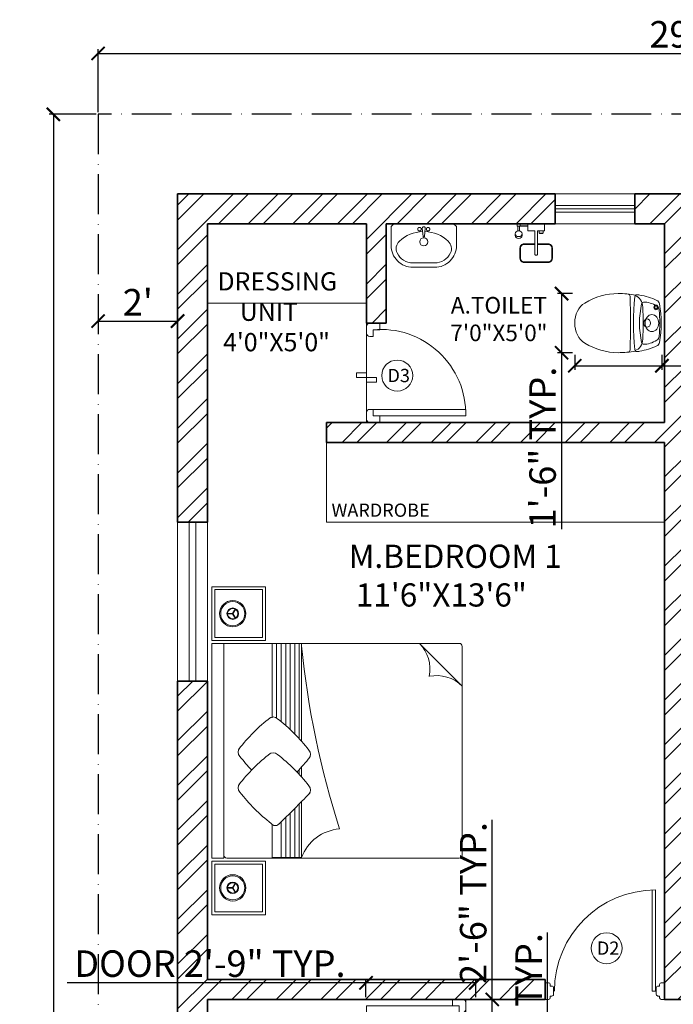
# Model space of a CAD drawing. Units: inches. Extents: x -15 to 1053, y -1 to 793.
# Tile 7 of 8: x 595 to 793, y 496 to 793. Entities that reach past the tile are written whole.
import ezdxf

# ---------------------------------------------------------------- set-up
doc = ezdxf.new("R2010")
doc.units = ezdxf.units.IN
doc.linetypes.add('ACAD_ISO10W100', pattern=[18, 12, -3, 0, -3])
for name, color, linetype, lineweight in [('00 FURNITURE', 15, 'Continuous', 15), ('A-ANNO-DIMS', 2, 'Continuous', 18), ('A-ANNO-TEXT', 7, 'Continuous', 18), ('A-AREA-IDEN', 7, 'Continuous', 18), ('A-DOOR', 4, 'Continuous', 18), ('A-FLOR-CASE', 5, 'Continuous', 18), ('A-FLOR-FIXT', 8, 'Continuous', 13), ('A-FURN', 8, 'Continuous', 13), ('A-GLAZ', 4, 'Continuous', 18), ('A-WALL', 7, 'Continuous', 35), ('A-WALL-PATT', 8, 'Continuous', 13), ('A_FUR 1', 5, 'Continuous', 5), ('C-PROP', 1, 'ACAD_ISO10W100', 25)]:
    doc.layers.add(name, color=color, linetype=linetype, lineweight=lineweight)
doc.styles.add('1-100DIM', font='txt', dxfattribs={"height": 0.3})
doc.styles.get("Standard").update_dxf_attribs({"font": 'arial.ttf'})
doc.dimstyles.new('ISO-25', dxfattribs={"dimtxt": 8, "dimasz": 4, "dimexe": 1.25, "dimexo": 0.625, "dimtad": 1, "dimdec": 0, "dimlunit": 4, "dimtxsty": 'Standard', "dimblk": 'ARCHTICK', "dimcen": 3, "dimadec": 0, "dimazin": 0, "dimtfac": 1, "dimtdec": 0, "dimtmove": 0, "dimatfit": 3, "dimldrblk": 'ARCHTICK', "dimfxl": 1, "dimarcsym": 0})

# ---------------------------------------------------------------- blocks, each defined once
blk = doc.blocks.new('_ArchTick')
at = {"color": 0, "linetype": 'ByBlock', "const_width": 0.15}
blk.add_lwpolyline([(-0.5, -0.5), (0.5, 0.5)], dxfattribs=at)
blk = doc.blocks.new('*D18')
at = {"layer": 'A-ANNO-DIMS', "color": 0, "lineweight": -2, "transparency": 16777216}
for p, q in [((619.07, 765.39), (619.07, 784.39)), ((967.07, 765.39), (967.07, 784.39)), ((619.07, 783.14), (967.07, 783.14))]:
    blk.add_line(p, q, dxfattribs=at)
at = {"layer": 'Defpoints', "color": 0, "transparency": 16777216}
for p in [(967.07, 783.14), (619.07, 764.76), (967.07, 764.76)]:
    blk.add_point(p, dxfattribs=at)
at = {"layer": 'A-ANNO-DIMS', "color": 0, "lineweight": -2, "transparency": 16777216, "xscale": 4, "yscale": 4, "zscale": 4, "rotation": 180}
blk.add_blockref('_ArchTick', (619.07, 783.14), dxfattribs=at)
at = {"layer": 'A-ANNO-DIMS', "color": 0, "lineweight": -2, "transparency": 16777216, "xscale": 4, "yscale": 4, "zscale": 4}
blk.add_blockref('_ArchTick', (967.07, 783.14), dxfattribs=at)
at = {"layer": 'A-ANNO-DIMS', "color": 0, "transparency": 16777216, "insert": (793.07, 787.85), "char_height": 8, "attachment_point": 5}
blk.add_mtext("29'", dxfattribs=at)
blk = doc.blocks.new('*D19')
at = {"layer": 'A-ANNO-DIMS', "color": 0, "lineweight": -2, "transparency": 16777216}
for p, q in [((618.45, 764.76), (604.32, 764.76)), ((605.57, 764.76), (605.57, 44.76)), ((618.45, 44.76), (604.32, 44.76))]:
    blk.add_line(p, q, dxfattribs=at)
at = {"layer": 'Defpoints', "color": 0, "transparency": 16777216}
for p in [(619.07, 764.76), (605.57, 44.76), (619.07, 44.76)]:
    blk.add_point(p, dxfattribs=at)
at = {"layer": 'A-ANNO-DIMS', "color": 0, "lineweight": -2, "transparency": 16777216, "xscale": 4, "yscale": 4, "zscale": 4}
for p, rotation in [((605.57, 764.76), 90), ((605.57, 44.76), 270)]:
    blk.add_blockref('_ArchTick', p, dxfattribs=dict(at, rotation=rotation))
at = {"layer": 'A-ANNO-DIMS', "color": 0, "transparency": 16777216, "insert": (600.86, 404.76), "char_height": 8, "attachment_point": 5, "rotation": 90}
blk.add_mtext("60'", dxfattribs=at)
blk = doc.blocks.new('ESTSET')
at = {"layer": 'A_FUR 1'}
for p, q in [((-10.44, 4.1), (-10.44, 32.1)), ((-8.44, 4.1), (-8.44, 32.1)), ((-36.44, 6.1), (-36.44, 3.1)), ((-34.44, 6.1), (-36.44, 6.1)), ((-34.44, 4.1), (-34.44, 6.1)), ((-34.44, 4.1), (-34.44, 6.1)), ((-8.44, 4.1), (-8.44, 6.1)), ((-8.44, 6.1), (-6.44, 6.1)), ((-8.44, 4.1), (-8.44, 6.1)), ((-6.44, 6.1), (-6.44, 3.1)), ((-32.44, 4.1), (-34.44, 4.1)), ((-32.44, 4.1), (-34.44, 4.1)), ((-32.44, 3.1), (-32.44, 4.1)), ((-10.44, 3.1), (-10.44, 4.1)), ((-10.44, 4.1), (-8.44, 4.1)), ((-10.44, 4.1), (-8.44, 4.1)), ((-6.44, 2.1), (-36.44, 2.1)), ((-35.44, 2.1), (-33.44, 2.1)), ((-7.44, 2.1), (-9.44, 2.1))]:
    blk.add_line(p, q, dxfattribs=at)
for points in [[(-21.44, 2.1), (-18.67, 2.1), (-18.67, 5.1), (-20.06, 5.1)], [(-20.06, 5.1), (-20.06, -0.91)], [(-21.44, 2.1), (-21.44, -0.91), (-20.06, -0.91)]]:
    blk.add_lwpolyline(points, dxfattribs=at)
for centre, radius, start, end in [((-8.91, 6.46), 25.64, 88.9606, 185.2816), ((-35.44, 3.1), 1, 180, 270), ((-33.44, 3.1), 1, 270, 0), ((-9.44, 3.1), 1, 180, 270), ((-7.44, 3.1), 1, 270, 0)]:
    blk.add_arc(centre, radius, start, end, dxfattribs=at)
blk = doc.blocks.new('DDD')
at = {"layer": '00 FURNITURE'}
for p, q in [((-12579.77, -15859.53), (-12579.77, -15829.05)), ((-12578.77, -15859.53), (-12578.77, -15829.03)), ((-12612.02, -15857.03), (-12612.02, -15862.03)), ((-12611.02, -15857.03), (-12612.02, -15857.03)), ((-12610.52, -15858.03), (-12610.52, -15857.53)), ((-12577.52, -15858.03), (-12577.52, -15857.53)), ((-12577.02, -15857.03), (-12576.02, -15857.03)), ((-12576.02, -15857.03), (-12576.02, -15862.03)), ((-12610.52, -15861.53), (-12610.52, -15861.03)), ((-12578.77, -15859.53), (-12579.77, -15859.53)), ((-12577.52, -15861.53), (-12577.52, -15861.03)), ((-12612.02, -15862.03), (-12611.02, -15862.03)), ((-12576.02, -15862.03), (-12577.02, -15862.03))]:
    blk.add_line(p, q, dxfattribs=at)
for points in [[(-12610.52, -15861.03), (-12610.02, -15861.03, 0.414214), (-12609.52, -15860.53), (-12609.52, -15858.53, 0.414214), (-12610.02, -15858.03), (-12610.52, -15858.03)], [(-12577.52, -15861.03), (-12578.02, -15861.03, -0.414214), (-12578.52, -15860.53), (-12578.52, -15858.53, -0.414214), (-12578.02, -15858.03), (-12577.52, -15858.03)]]:
    blk.add_lwpolyline(points, format="xyb", dxfattribs=at)
for centre, radius, start, end in [((-12578.77, -15859.53), 30.5, 90, 180), ((-12611.02, -15857.53), 0.5, 0, 90), ((-12577.02, -15857.53), 0.5, 90, 180), ((-12611.02, -15861.53), 0.5, 270, 0), ((-12577.02, -15861.53), 0.5, 180, 270)]:
    blk.add_arc(centre, radius, start, end, dxfattribs=at)
blk = doc.blocks.new('RGWTG')
at = {"layer": '00 FURNITURE'}
for p, q in [((578.23, 3473.51), (577.36, 3475.01)), ((578.23, 3473.58), (577.36, 3472.08)), ((578.36, 3473.58), (577.49, 3475.09)), ((578.36, 3473.51), (577.49, 3472)), ((578.29, 3473.62), (580.03, 3473.62)), ((578.29, 3473.47), (580.03, 3473.47)), ((521.93, 3464.58), (509.03, 3451.68)), ((509.03, 3422.63), (509.03, 3463.68)), ((509.93, 3464.58), (566.4, 3464.58)), ((557.53, 3463.84), (557.53, 3464.49)), ((557.53, 3464.49), (566.4, 3464.49)), ((558.2, 3464.49), (558.2, 3435.82)), ((559.57, 3464.49), (559.57, 3437.25)), ((560.94, 3464.49), (560.94, 3438.58)), ((562.3, 3464.49), (562.3, 3439.83)), ((563.67, 3464.49), (563.67, 3440.99)), ((565.04, 3464.49), (565.04, 3442.08)), ((566.4, 3464.58), (580.98, 3464.58)), ((566.4, 3464.49), (566.4, 3442.08)), ((566.4, 3464.49), (566.4, 3463.84)), ((580.98, 3464.58), (580.98, 3416.72)), ((558.2, 3426.48), (558.2, 3425.04)), ((509.03, 3400.68), (509.03, 3422.63)), ((558.2, 3416.13), (558.2, 3399.95)), ((580.98, 3416.72), (580.98, 3400.68)), ((559.57, 3414.75), (559.57, 3399.95)), ((560.94, 3413.39), (560.94, 3399.95)), ((562.3, 3412.04), (562.3, 3399.95)), ((563.67, 3410.72), (563.67, 3399.95)), ((580.08, 3399.78), (509.93, 3399.78)), ((557.53, 3399.95), (557.53, 3400.6)), ((566.4, 3399.95), (557.53, 3399.95)), ((566.4, 3400.6), (566.4, 3399.95)), ((578.23, 3390.78), (577.36, 3392.29)), ((578.36, 3390.86), (577.49, 3392.36)), ((578.23, 3390.86), (577.36, 3389.36)), ((578.36, 3390.78), (577.49, 3389.28)), ((578.29, 3390.9), (580.03, 3390.9)), ((578.29, 3390.74), (580.03, 3390.74))]:
    blk.add_line(p, q, dxfattribs=at)
for points in [[(568.43, 3465.48), (584.63, 3465.48), (584.63, 3481.68), (568.43, 3481.68)], [(569.33, 3466.38), (583.73, 3466.38), (583.73, 3480.78), (569.33, 3480.78)], [(580.98, 3399.78), (584.63, 3399.78), (584.63, 3464.58), (580.98, 3464.58)], [(568.43, 3398.88), (584.63, 3398.88), (584.63, 3382.68), (568.43, 3382.68)], [(569.33, 3397.98), (583.73, 3397.98), (583.73, 3383.58), (569.33, 3383.58)]]:
    blk.add_lwpolyline(points, close=True, dxfattribs=at)
for points in [[(566.52, 3464.49), (557.53, 3464.49), (557.53, 3435.08)], [(557.53, 3427.21), (557.53, 3424.3)], [(557.53, 3416.82), (557.53, 3399.95), (566.4, 3399.95), (566.4, 3409.94)]]:
    blk.add_lwpolyline(points, dxfattribs=at)
for centre, radius in [((578.29, 3473.54), 3.97), ((578.29, 3473.54), 3.63), ((578.29, 3473.54), 1.74), ((578.29, 3473.54), 1.56), ((578.29, 3390.82), 3.97), ((578.29, 3390.82), 3.63), ((578.29, 3390.82), 1.74), ((578.29, 3390.82), 1.56)]:
    blk.add_circle(centre, radius, dxfattribs=at)
for centre, radius, start, end in [((509.93, 3463.68), 0.9, 90, 180), ((529.65, 3456.88), 10.9, 135.0361, 191.9278), ((290.56, 3490.52), 268.3, 342.2214, 354.2925), ((516.73, 3443.97), 10.9, 78.0722, 134.9639), ((598.15, 3399.01), 54.32, 127.931, 142.069), ((566.05, 3440.57), 1.82, 45, 135), ((533.58, 3399.31), 54.32, 37.931, 52.069), ((556.59, 3431.11), 1.82, 135, 225), ((598.15, 3388.23), 54.32, 127.931, 142.069), ((566.05, 3429.78), 1.82, 45, 135), ((533.58, 3388.53), 54.32, 37.931, 52.069), ((574.84, 3431.77), 1.82, 315, 45), ((597.87, 3463.6), 54.32, 217.931, 224.141), ((533.28, 3463.88), 54.32, 316.32, 322.069), ((574.84, 3420.99), 1.82, 315, 45), ((556.59, 3420.33), 1.82, 135, 225), ((765.33, 3619.75), 290.45, 223.6069, 226.2326), ((533.28, 3453.1), 54.32, 307.931, 322.069), ((565.44, 3411.05), 1.47, 225.9674, 326.8337), ((545.02, 3395.29), 13.35, 20.4224, 85.5825), ((509.93, 3400.68), 0.9, 180, 270), ((580.08, 3400.68), 0.9, 270, 0)]:
    blk.add_arc(centre, radius, start, end, dxfattribs=at)
blk = doc.blocks.new('s_14')
at = {"extrusion": (0, 0, -1)}
for centre, major_axis, start_param, end_param in [((-0.2, -522.3), (652.4, -0.3), 4.476887, 4.947891), ((-0.2, -522.3), (652.4, -0.3), 4.476887, 4.947891), ((681.3, -278.7), (913.7, -0.4), 3.289642, 3.481728), ((681.3, -278.7), (913.7, -0.4), 3.289642, 3.481728), ((-143.1, -44.8), (39.1, 0), 3.481728, 4.476887), ((-143.1, -44.8), (39.1, 0), 3.481728, 4.476887), ((118.1, -139.4), (284.9, -0.1), 3.130806, 3.616946), ((-125.1, -42.1), (19.2, 0), 3.141593, 9.424778), ((-125.1, -42.1), (12.2, 0), 3.141593, 9.424778), ((-97.4, -50.5), (42.5, 0), 3.616946, 4.577347), ((-0.3, -624.1), (765.5, -0.4), 4.577347, 4.847431), ((0, -73.8), (67.1, 0), 3.141593, 9.424778), ((97.3, -50.6), (42.5, 0), -1.435755, -0.475353), ((-118.3, -139.3), (284.9, -0.1), -0.475353, 0.010787), ((143.1, -44.9), (39.1, 0), -1.335294, -0.340135), ((143.1, -44.9), (39.1, 0), -1.335294, -0.340135), ((-681.5, -278.1), (913.7, -0.4), -0.340135, -0.148049), ((-681.5, -278.1), (913.7, -0.4), -0.340135, -0.148049), ((-120.9, -224.6), (98.7, 0), 3.365215, 4.657014), ((-148.9, -141.6), (17.9, 0), 1.839297, 3.130806), ((0.1, 291.4), (579, -0.3), 1.302296, 1.839297), ((-0.9, -1969.6), (2281.8, -1.1), 4.657014, 4.767764), ((-0.1, -112.6), (32.9, 0), 3.141593, 9.424778), ((120.7, -224.8), (98.7, 0), -1.515421, -0.223622), ((148.8, -141.7), (17.9, 0), 0.010787, 1.302296), ((999.2, -341.8), (1233.1, -0.6), 3.141593, 3.282422), ((999.2, -341.8), (1233.1, -0.6), 3.141593, 3.282422), ((-87.1, -186.6), (136.8, -0.1), 3.032389, 3.289642), ((-87.1, -186.6), (136.8, -0.1), 3.032389, 3.289642), ((-207.2, -197.1), (16, 0), 1.680926, 3.032389), ((-207.2, -197.1), (16, 0), 1.680926, 3.032389), ((0.6, 1302.1), (1900.3, -0.9), 1.460666, 1.680926), ((0.6, 1302.1), (1900.3, -0.9), 1.460666, 1.680926), ((207, -197.3), (16, 0), 0.109204, 1.460666), ((207, -197.3), (16, 0), 0.109204, 1.460666), ((-999.6, -340.9), (1233.1, -0.6), -0.140829, 0), ((-999.6, -340.9), (1233.1, -0.6), -0.140829, 0), ((86.9, -186.7), (136.8, -0.1), -0.148049, 0.109204), ((86.9, -186.7), (136.8, -0.1), -0.148049, 0.109204), ((-210, -262.6), (19.7, 0), 3.222651, 4.658459), ((-1.6, -3375.8), (3914.3, -1.8), 4.658459, 4.766319), ((209.8, -262.8), (19.7, 0), -1.516867, -0.081058), ((526.7, -341.6), (760.5, -0.4), 2.693443, 3.141593), ((526.7, -341.6), (760.5, -0.4), 2.693443, 3.141593), ((-527, -341.1), (760.5, -0.4), 0, 0.44815), ((-527, -341.1), (760.5, -0.4), 0, 0.44815), ((-0.3, -544.1), (175.9, -0.1), 0.44815, 2.693443), ((-0.3, -544.1), (175.9, -0.1), 0.44815, 2.693443)]:
    blk.add_ellipse(centre, major_axis=major_axis, ratio=0.800511, start_param=start_param, end_param=end_param, dxfattribs=at)
blk = doc.blocks.new('s_46')
at = {"ltscale": 600}
h = blk.add_hatch(color=256, dxfattribs=at)
edge = h.paths.add_edge_path()
edge.add_line((13.5, 62), (14.2, 54.1))
edge.add_ellipse((4.2, 52.3), major_axis=(-10.1, 0), ratio=1, start_angle=540, end_angle=550.17546, ccw=False)
edge.add_arc((4.2, 52.3), 10.1, 270, 360, ccw=False)
edge.add_line((4.2, 42.2), (4.2, 41.3))
edge.add_line((4.2, 41.3), (11.9, 41.3))
edge.add_arc((4.2, 52.3), 13.4, 664.69813, 766.48477)
h.paths.add_polyline_path([(4.2, 41.3), (-3.4, 41.3, 0.152567), (4.2, 38.9)])
h.paths.add_polyline_path([(11.9, 41.3), (4.2, 41.3), (4.2, 38.9, 0.152567)])
h.paths.add_polyline_path([(-5.7, 54.1), (-5, 62, 0.475833), (-3.4, 41.3), (4.2, 41.3), (4.2, 42.2, -0.46724)])
for p, q in [((-5.9, 52.3), (-0.7, 110.5)), ((-5.9, 52.3), (-0.7, 110.5)), ((9.1, 110.5), (14.2, 54.1)), ((14.3, 52.3), (9.1, 110.5)), ((14.2, 54.1), (14.3, 52.3))]:
    blk.add_line(p, q, dxfattribs=at)
blk.add_lwpolyline([(-220.8, 171.3, -0.414214), (-70.8, 321.3), (79.2, 321.3, -0.414214), (229.2, 171.3), (229.2, 41.3), (209.2, 21.3), (-200.8, 21.3), (-220.8, 41.3)], format="xyb", close=True, dxfattribs=at)
blk.add_lwpolyline([(12.3, 75.4, 0.181638), (172.2, 141.5, 0.326351), (187.7, 222.7, 0.289814), (79.2, 291.3), (-70.8, 291.3, 0.289814), (-179.2, 222.7, 0.326351), (-163.8, 141.5, 0.181638), (-3.8, 75.4)], format="xyb", dxfattribs=at)
for points in [[(-16.8, 67.4), (-17, 67.5), (-17.2, 67.6), (-17.4, 67.6), (-17.6, 67.7), (-17.8, 67.8), (-18, 67.9), (-18.1, 68.1), (-18.2, 68.2), (-18.3, 68.4), (-18.4, 68.6), (-18.5, 68.8), (-18.7, 68.9), (-18.8, 69.1), (-18.9, 69.2), (-19.1, 69.3), (-19.3, 69.3), (-19.5, 69.3), (-19.7, 69.4), (-19.9, 69.4), (-20.1, 69.4), (-20.3, 69.4), (-20.5, 69.5), (-20.7, 69.6), (-20.8, 69.7), (-21, 69.9), (-21.1, 70), (-21.3, 70.2), (-21.4, 70.3), (-21.5, 70.4), (-21.7, 70.5), (-21.9, 70.5), (-22.1, 70.5), (-22.3, 70.5), (-22.5, 70.5), (-22.7, 70.4), (-22.9, 70.4), (-23.1, 70.4), (-23.3, 70.4), (-23.5, 70.5), (-23.7, 70.6), (-23.9, 70.7), (-24, 70.8), (-24.2, 70.9), (-24.4, 71), (-24.6, 71.1), (-24.7, 71.1), (-24.9, 71.1), (-25.1, 71), (-25.3, 71), (-25.5, 70.9), (-25.7, 70.8), (-25.9, 70.7), (-26.1, 70.6), (-26.3, 70.6), (-26.5, 70.6), (-26.7, 70.6), (-26.9, 70.7), (-27.1, 70.8), (-27.3, 70.8), (-27.5, 70.9), (-27.7, 70.9), (-27.8, 70.9), (-28, 70.8), (-28.2, 70.8), (-28.3, 70.6), (-28.5, 70.5), (-28.7, 70.4), (-28.9, 70.3), (-29.1, 70.2), (-29.3, 70.1), (-29.6, 70.1), (-29.9, 70.1), (-30.2, 70.1), (-30.5, 70), (-30.8, 69.8), (-31.1, 69.5), (-31.4, 69), (-31.6, 68.4), (-32.3, 68.5), (-32.8, 68.4), (-33.2, 68.3), (-33.5, 68.1), (-33.7, 67.8), (-33.9, 67.6), (-34, 67.3), (-34.1, 67.1), (-34.3, 66.9), (-34.5, 66.7), (-34.7, 66.6), (-34.9, 66.5), (-35.1, 66.4), (-35.2, 66.3), (-35.4, 66.2), (-35.5, 66), (-35.6, 65.9), (-35.6, 65.7), (-35.7, 65.5), (-35.7, 65.3), (-35.7, 65.1), (-35.8, 64.9), (-35.8, 64.7), (-35.9, 64.5), (-36, 64.3), (-36.2, 64.2), (-36.3, 64), (-36.5, 63.9), (-36.6, 63.8), (-36.8, 63.6), (-36.9, 63.5), (-37, 63.3), (-37, 63.1), (-37, 63), (-37, 62.8), (-37, 62.6), (-37, 62.3), (-37, 62.1), (-37, 61.9), (-37, 61.7), (-37.1, 61.5), (-37.2, 61.4), (-37.3, 61.2), (-37.4, 61), (-37.5, 60.8), (-37.6, 60.7), (-37.7, 60.5), (-37.8, 60.3), (-37.8, 60.1), (-37.7, 60), (-37.7, 59.8), (-37.6, 59.6), (-37.5, 59.4), (-37.4, 59.2), (-37.4, 59), (-37.4, 58.8), (-37.4, 58.6), (-37.4, 58.4), (-37.5, 58.2), (-37.6, 58), (-37.7, 57.8), (-37.7, 57.6), (-37.8, 57.4), (-37.8, 57.2), (-37.7, 57.1), (-37.6, 56.9), (-37.5, 56.7), (-37.4, 56.6), (-37.3, 56.4), (-37.2, 56.2), (-37.1, 56), (-37, 55.8), (-37, 55.6), (-37, 55.4), (-37, 55.2), (-37, 55), (-37, 54.8), (-37, 54.6), (-37, 54.4), (-37, 54.2), (-36.9, 54.1), (-36.8, 53.9), (-36.6, 53.8), (-36.5, 53.7), (-36.3, 53.5), (-36.2, 53.4), (-36, 53.2), (-35.9, 53.1), (-35.8, 52.9), (-35.8, 52.7), (-35.7, 52.5), (-35.7, 52.3), (-35.7, 52.1), (-35.6, 51.9), (-35.6, 51.7), (-35.5, 51.5), (-35.4, 51.4), (-35.2, 51.3), (-35.1, 51.2), (-34.9, 51.1), (-34.7, 51), (-34.5, 50.9), (-34.3, 50.8), (-34.2, 50.7), (-34, 50.5), (-33.9, 50.3), (-33.8, 50.1), (-33.8, 49.9), (-33.7, 49.8), (-33.6, 49.6), (-33.5, 49.4), (-33.4, 49.3), (-33.2, 49.2), (-33.1, 49.1), (-32.9, 49.1), (-32.7, 49), (-32.5, 49), (-32.2, 48.9), (-32.1, 48.9), (-31.9, 48.8), (-31.7, 48.7), (-31.6, 48.5), (-31.4, 48.3), (-31.3, 48.2), (-31.2, 48), (-31.1, 47.9), (-30.9, 47.7), (-30.8, 47.6), (-30.6, 47.6), (-30.4, 47.5), (-30.2, 47.5), (-30, 47.6), (-29.8, 47.6), (-29.6, 47.6), (-29.4, 47.6), (-29.2, 47.5), (-29, 47.4), (-28.8, 47.3), (-28.7, 47.2), (-28.5, 47.1), (-28.3, 46.9), (-28.2, 46.8), (-28, 46.7), (-27.8, 46.7), (-27.7, 46.7), (-27.5, 46.7), (-27.3, 46.7), (-27.1, 46.8), (-26.9, 46.9), (-26.7, 46.9), (-26.5, 47), (-26.3, 47), (-26.1, 46.9), (-25.9, 46.9), (-25.7, 46.8), (-25.5, 46.7), (-25.3, 46.6), (-25.1, 46.5), (-24.9, 46.5), (-24.7, 46.5), (-24.6, 46.5), (-24.4, 46.6), (-24.2, 46.7), (-24, 46.8), (-23.9, 46.9), (-23.7, 47), (-23.5, 47.1), (-23.3, 47.1), (-23.1, 47.2), (-22.9, 47.2), (-22.7, 47.1), (-22.5, 47.1), (-22.3, 47), (-22.1, 47), (-21.9, 47), (-21.7, 47.1), (-21.5, 47.1), (-21.4, 47.2), (-21.3, 47.4), (-21.1, 47.5), (-21, 47.7), (-20.8, 47.8), (-20.7, 48), (-20.5, 48.1), (-20.3, 48.1), (-20.1, 48.2), (-19.9, 48.2), (-19.7, 48.2), (-19.5, 48.2), (-19.3, 48.2), (-19.1, 48.3), (-18.9, 48.4), (-18.8, 48.5), (-18.7, 48.6), (-18.5, 48.8), (-18.4, 49), (-18.3, 49.2), (-18.2, 49.3), (-18.1, 49.5), (-18, 49.7), (-17.8, 49.8), (-17.6, 49.9), (-17.4, 49.9), (-17.2, 50), (-17, 50.1), (-16.8, 50.1), (-16.7, 50.2), (-16.5, 50.3), (-16.4, 50.5), (-16.3, 50.7), (-16.3, 50.8), (-16.2, 51), (-16.2, 51.3), (-16.1, 51.5), (-16, 51.6), (-15.9, 51.8), (-15.8, 52), (-15.6, 52.1), (-15.5, 52.2), (-15.3, 52.3), (-15.1, 52.4), (-15, 52.6), (-14.8, 52.7), (-14.7, 52.8), (-14.7, 53), (-14.6, 53.2), (-14.6, 53.4), (-14.6, 53.6), (-14.6, 53.8), (-14.6, 54), (-14.6, 54.2), (-14.5, 54.4), (-14.4, 54.6), (-14.3, 54.8), (-14.2, 54.9), (-14, 55.1), (-13.9, 55.2), (-13.7, 55.4), (-13.6, 55.5), (-13.6, 55.7), (-13.6, 55.9), (-13.6, 56.1), (-13.6, 56.3), (-13.7, 56.5), (-13.7, 56.7), (-13.8, 56.9), (-13.8, 57.1), (-13.8, 57.3), (-13.7, 57.5), (-13.7, 57.7), (-13.6, 57.9), (-13.5, 58.1), (-13.4, 58.2), (-13.3, 58.4), (-13.2, 58.6), (-13.2, 58.8), (-13.2, 59), (-13.3, 59.1), (-13.4, 59.3), (-13.5, 59.5), (-13.6, 59.7), (-13.7, 59.9), (-13.7, 60.1), (-13.8, 60.3), (-13.8, 60.5), (-13.8, 60.7), (-13.7, 60.9), (-13.7, 61.1), (-13.6, 61.3), (-13.6, 61.5), (-13.6, 61.7), (-13.6, 61.9), (-13.6, 62), (-13.7, 62.2), (-13.9, 62.3), (-14, 62.5), (-14.2, 62.6), (-14.3, 62.8), (-14.4, 63), (-14.5, 63.1), (-14.6, 63.3), (-14.6, 63.5), (-14.6, 63.8), (-14.6, 64), (-14.6, 64.2), (-14.6, 64.4), (-14.7, 64.6), (-14.7, 64.7), (-14.8, 64.9), (-15, 65), (-15.1, 65.1), (-15.3, 65.2), (-15.5, 65.3), (-15.6, 65.5), (-15.8, 65.6), (-15.9, 65.7), (-16, 65.9), (-16.1, 66.1), (-16.2, 66.3), (-16.2, 66.5), (-16.3, 66.7), (-16.3, 66.9), (-16.4, 67.1), (-16.5, 67.2), (-16.7, 67.3)], [(22.1, 61.1), (22, 61.3), (22, 61.5), (22, 61.7), (22, 61.9), (22.1, 62), (22.2, 62.2), (22.3, 62.3), (22.4, 62.5), (22.6, 62.6), (22.7, 62.8), (22.8, 63), (22.9, 63.1), (23, 63.3), (23, 63.5), (23, 63.8), (23, 64), (23, 64.2), (23, 64.4), (23.1, 64.6), (23.1, 64.7), (23.2, 64.9), (23.4, 65), (23.5, 65.1), (23.7, 65.2), (23.9, 65.3), (24.1, 65.5), (24.2, 65.6), (24.4, 65.7), (24.5, 65.9), (24.5, 66.1), (24.6, 66.3), (24.7, 66.5), (24.7, 66.7), (24.8, 66.9), (24.9, 67.1), (25, 67.2), (25.1, 67.3), (25.3, 67.4), (25.4, 67.5), (25.6, 67.6), (25.8, 67.6), (26, 67.7), (26.2, 67.8), (26.4, 67.9), (26.5, 68.1), (26.7, 68.2), (26.8, 68.4), (26.9, 68.6), (27, 68.8), (27.1, 68.9), (27.2, 69.1), (27.3, 69.2), (27.5, 69.3), (27.7, 69.3), (27.9, 69.3), (28.1, 69.4), (28.3, 69.4), (28.5, 69.4), (28.7, 69.4), (28.9, 69.5), (29.1, 69.6), (29.2, 69.7), (29.4, 69.9), (29.5, 70), (29.7, 70.2), (29.8, 70.3), (30, 70.4), (30.1, 70.5), (30.3, 70.5), (30.5, 70.5), (30.7, 70.5), (30.9, 70.5), (31.1, 70.4), (31.3, 70.4), (31.5, 70.4), (31.7, 70.4), (31.9, 70.5), (32.1, 70.6), (32.3, 70.7), (32.5, 70.8), (32.6, 70.9), (32.8, 71), (33, 71.1), (33.2, 71.1), (33.4, 71.1), (33.5, 71), (33.7, 71), (33.9, 70.9), (34.1, 70.8), (34.3, 70.7), (34.5, 70.6), (34.7, 70.6), (34.9, 70.6), (35.1, 70.6), (35.3, 70.7), (35.5, 70.8), (35.7, 70.8), (35.9, 70.9), (36.1, 70.9), (36.3, 70.9), (36.4, 70.8), (36.6, 70.8), (36.8, 70.6), (36.9, 70.5), (37.1, 70.4), (37.3, 70.3), (37.5, 70.2), (37.8, 70.1), (38, 70.1), (38.3, 70.1), (38.6, 70.1), (38.9, 70), (39.2, 69.8), (39.5, 69.5), (39.8, 69), (40.1, 68.4), (40.7, 68.5), (41.3, 68.4), (41.7, 68.3), (42, 68.1), (42.2, 67.8), (42.3, 67.6), (42.4, 67.3), (42.6, 67.1), (42.7, 66.9), (42.9, 66.7), (43.1, 66.6), (43.3, 66.5), (43.5, 66.4), (43.6, 66.3), (43.8, 66.2), (43.9, 66), (44, 65.9), (44.1, 65.7), (44.1, 65.5), (44.1, 65.3), (44.2, 65.1), (44.2, 64.9), (44.2, 64.7), (44.3, 64.5), (44.4, 64.3), (44.6, 64.2), (44.7, 64), (44.9, 63.9), (45.1, 63.8), (45.2, 63.6), (45.3, 63.5), (45.4, 63.3), (45.5, 63.1), (45.5, 63), (45.5, 62.8), (45.4, 62.6), (45.4, 62.3), (45.4, 62.1), (45.4, 61.9), (45.4, 61.7), (45.5, 61.5), (45.6, 61.4), (45.7, 61.2), (45.8, 61), (46, 60.8), (46.1, 60.7), (46.1, 60.5), (46.2, 60.3), (46.2, 60.1), (46.1, 60), (46.1, 59.8), (46, 59.6), (45.9, 59.4), (45.9, 59.2), (45.8, 59), (45.8, 58.8), (45.8, 58.6), (45.9, 58.4), (45.9, 58.2), (46, 58), (46.1, 57.8), (46.1, 57.6), (46.2, 57.4), (46.2, 57.2), (46.1, 57.1), (46.1, 56.9), (46, 56.7), (45.8, 56.6), (45.7, 56.4), (45.6, 56.2), (45.5, 56), (45.4, 55.8), (45.4, 55.6), (45.4, 55.4), (45.4, 55.2), (45.4, 55), (45.5, 54.8), (45.5, 54.6), (45.5, 54.4), (45.4, 54.2), (45.3, 54.1), (45.2, 53.9), (45.1, 53.8), (44.9, 53.7), (44.7, 53.5), (44.6, 53.4), (44.4, 53.2), (44.3, 53.1), (44.2, 52.9), (44.2, 52.7), (44.2, 52.5), (44.1, 52.3), (44.1, 52.1), (44.1, 51.9), (44, 51.7), (43.9, 51.5), (43.8, 51.4), (43.6, 51.3), (43.5, 51.2), (43.3, 51.1), (43.1, 51), (42.9, 50.9), (42.7, 50.8), (42.6, 50.7), (42.5, 50.5), (42.4, 50.3), (42.3, 50.1), (42.2, 49.9), (42.1, 49.8), (42, 49.6), (41.9, 49.4), (41.8, 49.3), (41.7, 49.2), (41.5, 49.1), (41.3, 49.1), (41.1, 49), (40.9, 49), (40.7, 48.9), (40.5, 48.9), (40.3, 48.8), (40.1, 48.7), (40, 48.5), (39.9, 48.3), (39.7, 48.2), (39.6, 48), (39.5, 47.9), (39.4, 47.7), (39.2, 47.6), (39, 47.6), (38.8, 47.5), (38.6, 47.5), (38.4, 47.6), (38.2, 47.6), (38, 47.6), (37.8, 47.6), (37.6, 47.5), (37.4, 47.4), (37.2, 47.3), (37.1, 47.2), (36.9, 47.1), (36.8, 46.9), (36.6, 46.8), (36.4, 46.7), (36.3, 46.7), (36.1, 46.7), (35.9, 46.7), (35.7, 46.7), (35.5, 46.8), (35.3, 46.9), (35.1, 46.9), (34.9, 47), (34.7, 47), (34.5, 46.9), (34.3, 46.9), (34.1, 46.8), (33.9, 46.7), (33.7, 46.6), (33.5, 46.5), (33.4, 46.5), (33.2, 46.5), (33, 46.5), (32.8, 46.6), (32.6, 46.7), (32.5, 46.8), (32.3, 46.9), (32.1, 47), (31.9, 47.1), (31.7, 47.1), (31.5, 47.2), (31.3, 47.2), (31.1, 47.1), (30.9, 47.1), (30.7, 47), (30.5, 47), (30.3, 47), (30.1, 47.1), (30, 47.1), (29.8, 47.2), (29.7, 47.4), (29.5, 47.5), (29.4, 47.7), (29.2, 47.8), (29.1, 48), (28.9, 48.1), (28.7, 48.1), (28.5, 48.2), (28.3, 48.2), (28.1, 48.2), (27.9, 48.2), (27.7, 48.2), (27.5, 48.3), (27.3, 48.4), (27.2, 48.5), (27.1, 48.6), (27, 48.8), (26.9, 49), (26.8, 49.2), (26.7, 49.3), (26.5, 49.5), (26.4, 49.7), (26.2, 49.8), (26, 49.9), (25.8, 49.9), (25.6, 50), (25.4, 50.1), (25.3, 50.1), (25.1, 50.2), (25, 50.3), (24.9, 50.5), (24.8, 50.7), (24.7, 50.8), (24.7, 51), (24.6, 51.3), (24.5, 51.5), (24.5, 51.6), (24.4, 51.8), (24.2, 52), (24.1, 52.1), (23.9, 52.2), (23.7, 52.3), (23.5, 52.4), (23.4, 52.6), (23.2, 52.7), (23.1, 52.8), (23.1, 53), (23, 53.2), (23, 53.4), (23, 53.6), (23, 53.8), (23, 54), (23, 54.2), (22.9, 54.4), (22.8, 54.6), (22.7, 54.8), (22.6, 54.9), (22.4, 55.1), (22.3, 55.2), (22.2, 55.4), (22.1, 55.5), (22, 55.7), (22, 55.9), (22, 56.1), (22, 56.3), (22.1, 56.5), (22.1, 56.7), (22.2, 56.9), (22.2, 57.1), (22.2, 57.3), (22.2, 57.5), (22.1, 57.7), (22, 57.9), (21.9, 58.1), (21.8, 58.2), (21.7, 58.4), (21.6, 58.6), (21.6, 58.8), (21.6, 59), (21.7, 59.1), (21.8, 59.3), (21.9, 59.5), (22, 59.7), (22.1, 59.9), (22.2, 60.1), (22.2, 60.3), (22.2, 60.5), (22.2, 60.7), (22.1, 60.9)]]:
    blk.add_lwpolyline(points, close=True, dxfattribs=at)
blk.add_circle((4.2, 146.3), 28, dxfattribs=at)
for centre, radius, start, end in [((4.2, 108.2), 5.42, 24.6783, 155.3217), ((4.2, 52.3), 10.1, 169.82454, 0)]:
    blk.add_arc(centre, radius, start, end, dxfattribs=at)
for centre, major_axis, ratio, start_param, end_param in [((4.2, 110.5), (-4.93, 0), 0.641024, 3.141593, 6.283185), ((4.2, 52.3), (-10.1, 0), 1, 6.10559, 9.602373)]:
    blk.add_ellipse(centre, major_axis=major_axis, ratio=ratio, start_param=start_param, end_param=end_param, dxfattribs=at)
blk = doc.blocks.new('A$C7A0926BE')
for p, q in [((-6.55, 0), (-5.57, 0)), ((-6.55, -0.65), (-6.55, 0)), ((-5.57, 0), (-5.57, -0.65)), ((-2.89, 0), (-2.89, -2.29)), ((2.89, 0), (-2.89, 0)), ((2.89, -2.29), (2.89, 0)), ((-7.32, -3.29), (-7.32, -3.94)), ((-5.57, -0.65), (-6.55, -0.65)), ((-6.34, -0.65), (-5.74, -0.65)), ((-6.34, -2.33), (-6.34, -0.65)), ((-5.74, -2.33), (-6.34, -2.33)), ((-5.74, -0.65), (-5.74, -2.33)), ((-5.57, -0.28), (-2.89, -0.56)), ((-5.57, -0.65), (-2.89, -0.94)), ((-4.84, -3.94), (-4.85, -3.29)), ((-2.89, -2.29), (-0.45, -2.29)), ((0.39, -2.29), (2.89, -2.29)), ((1.04, -2.29), (1.04, -3.12)), ((2.37, -2.29), (1.04, -2.29)), ((1.04, -3.12), (2.37, -3.12)), ((1.13, -3.12), (1.13, -3.23)), ((2.3, -3.12), (1.13, -3.12)), ((1.13, -3.23), (2.3, -3.23)), ((2.3, -3.23), (2.3, -3.12)), ((2.37, -3.12), (2.37, -2.29))]:
    blk.add_line(p, q)
at = {"ltscale": 100}
for p, q in [((-0.45, -10.48), (-0.45, -2.29)), ((0.39, -10.48), (0.39, -2.29)), ((0.18, -10.69), (-0.24, -10.69))]:
    blk.add_line(p, q, dxfattribs=at)
for points in [[(-0.45, -6.79), (-4.23, -6.79, 0.414214), (-5.63, -8.19), (-5.63, -11.8, 0.414214), (-4.23, -13.2), (4.17, -13.2, 0.414214), (5.57, -11.8), (5.57, -8.19, 0.414214), (4.17, -6.79), (0.39, -6.79)], [(-0.45, -7), (-4.23, -7, 0.414214), (-5.42, -8.19), (-5.42, -11.8, 0.414214), (-4.23, -12.99), (4.17, -12.99, 0.414214), (5.36, -11.8), (5.36, -8.19, 0.414214), (4.17, -7), (0.39, -7)]]:
    blk.add_lwpolyline(points, format="xyb", dxfattribs=at)
for centre, start, end in [((-0.24, -10.48), 180, 270), ((0.18, -10.48), 270, 0)]:
    blk.add_arc(centre, 0.21, start, end, dxfattribs=at)
at = {"extrusion": (0, 0, -1)}
blk.add_ellipse((-6.08, -3.29), major_axis=(-1.24, 0), ratio=0.790849, dxfattribs=at)
blk.add_ellipse((-6.08, -3.94), major_axis=(-1.24, 0), ratio=0.790849, start_param=3.141593, end_param=6.283185, dxfattribs=at)
blk = doc.blocks.new('*D24')
at = {"layer": 'A-ANNO-DIMS', "color": 0, "lineweight": -2, "transparency": 16777216}
for p, q in [((619.07, 702.4), (619.07, 701.14)), ((619.07, 702.39), (643.07, 702.39)), ((643.07, 702.4), (643.07, 701.14))]:
    blk.add_line(p, q, dxfattribs=at)
at = {"layer": 'Defpoints', "color": 0, "transparency": 16777216}
for p in [(619.07, 703.03), (643.07, 703.03), (643.07, 702.39)]:
    blk.add_point(p, dxfattribs=at)
at = {"layer": 'A-ANNO-DIMS', "color": 0, "lineweight": -2, "transparency": 16777216, "xscale": 4, "yscale": 4, "zscale": 4, "rotation": 180}
blk.add_blockref('_ArchTick', (619.07, 702.39), dxfattribs=at)
at = {"layer": 'A-ANNO-DIMS', "color": 0, "lineweight": -2, "transparency": 16777216, "xscale": 4, "yscale": 4, "zscale": 4}
blk.add_blockref('_ArchTick', (643.07, 702.39), dxfattribs=at)
at = {"layer": 'A-ANNO-DIMS', "color": 0, "transparency": 16777216, "insert": (631.07, 707.03), "char_height": 8, "attachment_point": 5}
blk.add_mtext("2'", dxfattribs=at)
blk = doc.blocks.new('*D36')
at = {"layer": 'A-ANNO-DIMS', "color": 0, "lineweight": -2, "transparency": 16777216}
for p, q in [((699.94, 502.73), (609.69, 502.73)), ((699.94, 498.39), (699.94, 503.98)), ((733.08, 502.73), (699.94, 502.73)), ((733.08, 498.39), (733.08, 503.98))]:
    blk.add_line(p, q, dxfattribs=at)
at = {"layer": 'Defpoints', "color": 0, "transparency": 16777216}
for p in [(699.94, 502.73), (699.94, 497.76), (733.08, 497.76)]:
    blk.add_point(p, dxfattribs=at)
at = {"layer": 'A-ANNO-DIMS', "color": 0, "lineweight": -2, "transparency": 16777216, "xscale": 4, "yscale": 4, "zscale": 4, "rotation": 180}
blk.add_blockref('_ArchTick', (699.94, 502.73), dxfattribs=at)
at = {"layer": 'A-ANNO-DIMS', "color": 0, "lineweight": -2, "transparency": 16777216, "xscale": 4, "yscale": 4, "zscale": 4}
blk.add_blockref('_ArchTick', (733.08, 502.73), dxfattribs=at)
at = {"layer": 'A-ANNO-DIMS', "color": 0, "transparency": 16777216, "insert": (652.82, 507.5), "char_height": 8, "attachment_point": 5}
blk.add_mtext('DOOR 2\'-9" TYP.', dxfattribs=at)
blk = doc.blocks.new('*D37')
at = {"layer": 'A-ANNO-DIMS', "color": 0, "lineweight": -2, "transparency": 16777216}
for p, q in [((738.05, 497.76), (738.05, 551.91)), ((733.7, 497.76), (739.3, 497.76)), ((738.05, 467.76), (738.05, 497.76)), ((733.7, 467.76), (739.3, 467.76))]:
    blk.add_line(p, q, dxfattribs=at)
at = {"layer": 'Defpoints', "color": 0, "transparency": 16777216}
for p in [(733.08, 497.76), (738.05, 497.76), (733.08, 467.76)]:
    blk.add_point(p, dxfattribs=at)
at = {"layer": 'A-ANNO-DIMS', "color": 0, "lineweight": -2, "transparency": 16777216, "xscale": 4, "yscale": 4, "zscale": 4}
for p, rotation in [((738.05, 497.76), 90), ((738.05, 467.76), 270)]:
    blk.add_blockref('_ArchTick', p, dxfattribs=dict(at, rotation=rotation))
at = {"layer": 'A-ANNO-DIMS', "color": 0, "transparency": 16777216, "insert": (733.34, 526.84), "char_height": 8, "attachment_point": 5, "rotation": 90}
blk.add_mtext('2\'-6" TYP.', dxfattribs=at)
blk = doc.blocks.new('*D38')
at = {"layer": 'A-ANNO-DIMS', "color": 0, "lineweight": -2, "transparency": 16777216}
for p, q in [((762.94, 692.23), (762.94, 687.66)), ((789.26, 692.23), (789.26, 687.66)), ((762.94, 688.91), (789.26, 688.91)), ((789.26, 688.91), (883.97, 688.91))]:
    blk.add_line(p, q, dxfattribs=at)
at = {"layer": 'Defpoints', "color": 0, "transparency": 16777216}
for p in [(762.94, 692.85), (789.26, 692.85), (789.26, 688.91)]:
    blk.add_point(p, dxfattribs=at)
at = {"layer": 'A-ANNO-DIMS', "color": 0, "lineweight": -2, "transparency": 16777216, "xscale": 4, "yscale": 4, "zscale": 4, "rotation": 180}
blk.add_blockref('_ArchTick', (762.94, 688.91), dxfattribs=at)
at = {"layer": 'A-ANNO-DIMS', "color": 0, "lineweight": -2, "transparency": 16777216, "xscale": 4, "yscale": 4, "zscale": 4}
blk.add_blockref('_ArchTick', (789.26, 688.91), dxfattribs=at)
at = {"layer": 'A-ANNO-DIMS', "color": 0, "transparency": 16777216, "insert": (838.61, 693.67), "char_height": 8, "attachment_point": 5}
blk.add_mtext('WC 2\'-2 1/2" TYP.', dxfattribs=at)
blk = doc.blocks.new('*D39')
at = {"layer": 'A-ANNO-DIMS', "color": 0, "lineweight": -2, "transparency": 16777216}
for p, q in [((762.31, 710.69), (757.74, 710.69)), ((758.99, 710.69), (758.99, 692.85)), ((762.31, 692.85), (757.74, 692.85)), ((758.99, 692.85), (758.99, 639.59))]:
    blk.add_line(p, q, dxfattribs=at)
at = {"layer": 'Defpoints', "color": 0, "transparency": 16777216}
for p in [(762.94, 710.69), (758.99, 692.85), (762.94, 692.85)]:
    blk.add_point(p, dxfattribs=at)
at = {"layer": 'A-ANNO-DIMS', "color": 0, "lineweight": -2, "transparency": 16777216, "xscale": 4, "yscale": 4, "zscale": 4}
for p, rotation in [((758.99, 710.69), 90), ((758.99, 692.85), 270)]:
    blk.add_blockref('_ArchTick', p, dxfattribs=dict(at, rotation=rotation))
at = {"layer": 'A-ANNO-DIMS', "color": 0, "transparency": 16777216, "insert": (754.28, 664.22), "char_height": 8, "attachment_point": 5, "rotation": 90}
blk.add_mtext('1\'-6" TYP.', dxfattribs=at)
blk = doc.blocks.new('*D41')
at = {"layer": 'A-ANNO-DIMS', "color": 0, "lineweight": -2, "transparency": 16777216}
for p, q in [((754.73, 464.71), (754.73, 517.97)), ((752.39, 464.71), (755.98, 464.71)), ((754.73, 451.54), (754.73, 464.71)), ((752.39, 451.54), (755.98, 451.54))]:
    blk.add_line(p, q, dxfattribs=at)
at = {"layer": 'Defpoints', "color": 0, "transparency": 16777216}
for p in [(751.77, 464.71), (754.73, 464.71), (751.77, 451.54)]:
    blk.add_point(p, dxfattribs=at)
at = {"layer": 'A-ANNO-DIMS', "color": 0, "lineweight": -2, "transparency": 16777216, "xscale": 4, "yscale": 4, "zscale": 4}
for p, rotation in [((754.73, 464.71), 90), ((754.73, 451.54), 270)]:
    blk.add_blockref('_ArchTick', p, dxfattribs=dict(at, rotation=rotation))
at = {"layer": 'A-ANNO-DIMS', "color": 0, "transparency": 16777216, "insert": (750.08, 493.34), "char_height": 8, "attachment_point": 5, "rotation": 90}
blk.add_mtext('1\'-1" TYP.', dxfattribs=at)

msp = doc.modelspace()

# ---------------------------------------------------------------- hatches: boundary and pattern name
at = {"layer": 'A-WALL-PATT'}
h = msp.add_hatch(dxfattribs=at)
h.set_pattern_fill('ANSI32', color=256)
h.paths.add_polyline_path([(754.07, 502.76), (754.07, 503.76), (652.07, 503.76), (652.07, 593.76), (643.07, 593.76), (643.07, 485.76), (652.07, 485.76), (652.07, 497.76), (754.07, 497.76)])
h.paths.add_polyline_path([(754.07, 449.76), (730.07, 449.76), (730.07, 467.76), (724.07, 467.76), (724.07, 449.76), (652.07, 449.76), (652.07, 461.76), (643.07, 461.76), (643.07, 374.76), (652.07, 374.76), (652.07, 443.76), (754.07, 443.76)])
h.paths.add_polyline_path([(757.07, 740.76), (643.07, 740.76), (643.07, 641.76), (652.07, 641.76), (652.07, 731.76), (700.07, 731.76), (700.07, 701.76), (706.07, 701.76), (706.07, 731.76), (757.07, 731.76)])
h.paths.add_polyline_path([(943.07, 740.76), (781.07, 740.76), (781.07, 731.76), (790.07, 731.76), (790.07, 671.76), (688.07, 671.76), (688.07, 665.76), (790.07, 665.76), (790.07, 497.76), (796.07, 497.76), (796.07, 502.76), (796.07, 731.76), (844.07, 731.76), (844.07, 701.76), (850.07, 701.76), (850.07, 731.76), (934.07, 731.76), (934.07, 713.76), (943.07, 713.76)])
h.paths.add_polyline_path([(943.07, 689.76), (934.07, 689.76), (934.07, 671.76), (832.07, 671.76), (832.07, 665.76), (934.07, 665.76), (934.07, 608.76), (943.07, 608.76)], flags=17)
h.paths.add_polyline_path([(943.07, 560.76), (934.07, 560.76), (934.07, 503.76), (832.07, 503.76), (832.07, 497.76), (934.07, 497.76), (934.07, 488.76), (943.07, 488.76)])
h.paths.add_polyline_path([(796.07, 449.76), (790.07, 449.76), (790.07, 444.76), (790.07, 326.76), (643.07, 326.76), (643.07, 320.76), (724.07, 320.76), (724.07, 266.76), (730.07, 266.76), (730.07, 320.76), (790.07, 320.76), (790.07, 272.76), (760.07, 272.76), (760.07, 266.76), (796.07, 266.76)])
h.paths.add_polyline_path([(652.07, 266.76), (688.07, 266.76), (688.07, 271.76), (688.07, 272.76), (643.07, 272.76), (643.07, 230.76), (652.07, 230.76)])
h.paths.add_polyline_path([(652.07, 182.76), (643.07, 182.76), (643.07, 146.76), (619.07, 146.76), (619.07, 44.76), (799.07, 44.76), (799.07, 53.76), (628.07, 53.76), (628.07, 137.76), (808.07, 137.76), (808.07, 146.76), (796.07, 146.76), (796.07, 218.76), (802.07, 218.76), (802.07, 224.76), (790.07, 224.76), (790.07, 146.76), (652.07, 146.76)])
h.paths.add_polyline_path([(886.07, 141.37), (886.07, 146.76), (850.07, 146.76), (850.07, 224.76), (838.07, 224.76), (838.07, 222.06), (838.07, 218.76), (844.07, 218.76), (844.07, 146.76), (832.07, 146.76), (832.07, 137.76), (886.07, 137.76)])
h.paths.add_polyline_path([(943.07, 176.76), (934.07, 176.76), (934.07, 137.76), (943.07, 137.76)])
h.paths.add_polyline_path([(943.07, 440.76), (934.07, 440.76), (934.07, 224.76), (943.07, 224.76)])

# ---------------------------------------------------------------- linework, layer by layer
at = {"layer": 'A-ANNO-TEXT'}
for centre in [(709.37, 685.95), (772.58, 513.2)]:
    msp.add_circle(centre, 4.67, dxfattribs=at)
at = {"layer": 'A-FLOR-CASE'}
for p, q in [((700.07, 707.76), (652.07, 707.76)), ((688.07, 665.76), (688.07, 641.76)), ((688.07, 641.76), (790.07, 641.76))]:
    msp.add_line(p, q, dxfattribs=at)
at = {"layer": 'A-GLAZ'}
for p, q in [((781.07, 737.26), (757.07, 737.26)), ((781.07, 736.26), (757.07, 736.26)), ((781.07, 735.26), (757.07, 735.26)), ((643.07, 641.76), (643.07, 593.76)), ((646.57, 641.76), (646.57, 593.76)), ((648.57, 641.76), (648.57, 593.76)), ((652.07, 641.76), (652.07, 593.76))]:
    msp.add_line(p, q, dxfattribs=at)
msp.add_lwpolyline([(757.07, 740.76), (757.07, 731.76), (781.07, 731.76), (781.07, 740.76)], close=True, dxfattribs=at)
at = {"layer": 'A-WALL'}
for p, q in [((643.07, 740.76), (643.07, 641.76)), ((757.07, 740.76), (643.07, 740.76)), ((757.07, 740.76), (757.07, 731.76)), ((943.07, 740.76), (781.07, 740.76)), ((781.07, 740.76), (781.07, 731.76)), ((652.07, 731.76), (652.07, 641.76)), ((700.07, 731.76), (652.07, 731.76)), ((700.07, 731.76), (700.07, 701.76)), ((757.07, 731.76), (706.07, 731.76)), ((706.07, 731.76), (706.07, 701.76)), ((790.07, 731.76), (781.07, 731.76)), ((790.07, 731.76), (790.07, 671.76)), ((706.07, 701.76), (700.07, 701.76)), ((790.07, 671.76), (688.07, 671.76)), ((688.07, 671.76), (688.07, 665.76)), ((790.07, 665.76), (688.07, 665.76)), ((790.07, 665.76), (790.07, 497.76)), ((643.07, 641.76), (652.07, 641.76)), ((643.07, 593.76), (652.07, 593.76)), ((643.07, 593.76), (643.07, 485.76)), ((652.07, 593.76), (652.07, 503.76)), ((652.07, 503.76), (754.07, 503.76)), ((754.07, 503.76), (754.07, 497.76)), ((652.07, 497.76), (754.07, 497.76)), ((652.07, 497.76), (652.07, 485.76)), ((790.07, 497.76), (796.07, 497.76))]:
    msp.add_line(p, q, dxfattribs=at)
at = {"layer": 'C-PROP'}
for p, q in [((967.07, 764.76), (619.07, 764.76)), ((619.07, 764.76), (619.07, 44.76))]:
    msp.add_line(p, q, dxfattribs=at)

# ---------------------------------------------------------------- block references
at = {"layer": 'A-DOOR'}
for p, rotation in [((697.98, 665.32), 270), ((732.17, 504.21), 90.00000000000003)]:
    msp.add_blockref('ESTSET', p, dxfattribs=dict(at, rotation=rotation))
msp.add_blockref('DDD', (13366.1, 16359.79), dxfattribs=at)
at = {"layer": 'A-FLOR-FIXT'}
for name, p, xscale, yscale, zscale, rotation in [('s_46', (717.57, 732.7), 0.0438792252617072, 0.0438792252617072, 0.0438792252617072, 180), ('s_14', (789.07, 701.76), 0.0381558672165204, 0.0381558672165204, 0.0381558672165204, 270)]:
    msp.add_blockref(name, p, dxfattribs=dict(at, xscale=xscale, yscale=yscale, zscale=zscale, rotation=rotation))
at = {"layer": 'A-FLOR-FIXT', "extrusion": (0, 0, -1), "xscale": -0.8732967133751344, "yscale": 0.8732967133751344, "zscale": -0.8732967133751344}
msp.add_blockref('A$C7A0926BE', (-751.34, 731.61), dxfattribs=at)
at = {"layer": 'A-FURN', "xscale": -1}
msp.add_blockref('RGWTG', (1238, -2859.42), dxfattribs=at)

# ---------------------------------------------------------------- texts
at = {"layer": 'A-ANNO-TEXT', "char_height": 4, "attachment_point": 1}
for s, width, insert in [('D3', 8.4888, (706.43, 687.97)), ('WARDROBE', 23.2678, (689.53, 647.34)), ('D2', 8.4888, (769.64, 515.22))]:
    msp.add_mtext_dynamic_manual_height_columns(s, width=width, gutter_width=12.5, heights=[0], dxfattribs=dict(at, insert=insert))
at = {"layer": 'A-AREA-IDEN', "insert": (655.13, 717.11), "char_height": 8, "attachment_point": 1}
msp.add_mtext_dynamic_manual_height_columns('{\\H0.6875x;DRESSING\\P    UNIT\\P 4\'0"X5\'0" \\H1.18182x;    }  ', width=58.9878, gutter_width=0, heights=[37.04], dxfattribs=at)
at = {"layer": 'A-AREA-IDEN', "attachment_point": 1, "style": '1-100DIM'}
for s, width, insert, char_height in [('\\pxqc;{\\f@Malgun Gothic|b0|i0|c0|p34;A.TOILET\\P7\'0"X5\'0"}', 44.4016, (717.86, 709.66), 5), ('{\\f@Malgun Gothic|b0|i0|c0|p34;M.BEDROOM 1\\P 11\'6"X13\'6"}', 74.3652, (694.73, 634.93), 7)]:
    msp.add_mtext_dynamic_manual_height_columns(s, width=width, gutter_width=15.85, heights=[0], dxfattribs=dict(at, insert=insert, char_height=char_height))

# ---------------------------------------------------------------- dimensions: what is measured, and where the dimension line sits
at = {"layer": 'A-ANNO-DIMS'}
for base, p1, p2, picture, middle in [((967.07, 783.14), (619.07, 764.76), (967.07, 764.76), '*D18', (793.07, 787.85)), ((643.07, 702.39), (619.07, 703.03), (643.07, 703.03), '*D24', (631.07, 707.03))]:
    dim = msp.add_linear_dim(base=base, p1=p1, p2=p2, dimstyle='ISO-25', override={"dimclrd": 0, "dimclre": 0, "dimclrt": 0}, dxfattribs=at)
    dim.commit()
    dim.dimension.update_dxf_attribs({"geometry": picture, "text_midpoint": middle})
dim = msp.add_linear_dim(base=(605.57, 44.76), p1=(619.07, 764.76), p2=(619.07, 44.76), angle=90, dimstyle='ISO-25', override={"dimclrd": 0, "dimclre": 0, "dimclrt": 0}, dxfattribs=at)
dim.commit()
dim.dimension.update_dxf_attribs({"geometry": '*D19', "text_midpoint": (600.86, 404.76)})
dim = msp.add_linear_dim(base=(789.26, 688.91), p1=(762.94, 692.85), p2=(789.26, 692.85), text='WC <> TYP.', dimstyle='ISO-25', override={"dimdec": 1, "dimrnd": 0, "dimzin": 1, "dimlunit": 4, "dimfrac": 2}, dxfattribs=at)
dim.commit()
dim.dimension.update_dxf_attribs({"geometry": '*D38', "text_midpoint": (838.61, 693.67)})
for base, p1, p2, angle, text, picture, middle in [((758.99, 692.85), (762.94, 710.69), (762.94, 692.85), 270, '<> TYP.', '*D39', (754.28, 664.22)), ((738.05, 497.76), (733.08, 467.76), (733.08, 497.76), 90, '<> TYP.', '*D37', (733.34, 526.84)), ((699.94, 502.73), (733.08, 497.76), (699.94, 497.76), 180, 'DOOR <> TYP.', '*D36', (652.82, 507.5)), ((754.73, 464.71), (751.77, 451.54), (751.77, 464.71), 90, '<> TYP.', '*D41', (750.08, 493.34))]:
    dim = msp.add_linear_dim(base=base, p1=p1, p2=p2, angle=angle, text=text, dimstyle='ISO-25', override={"dimdec": 1, "dimrnd": 0, "dimzin": 1, "dimlunit": 4, "dimfrac": 2}, dxfattribs=at)
    dim.commit()
    dim.dimension.update_dxf_attribs({"geometry": picture, "text_midpoint": middle})

doc.saveas('drawing.dxf')
